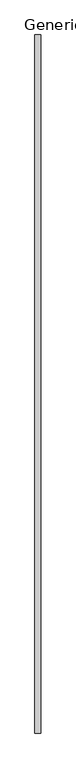
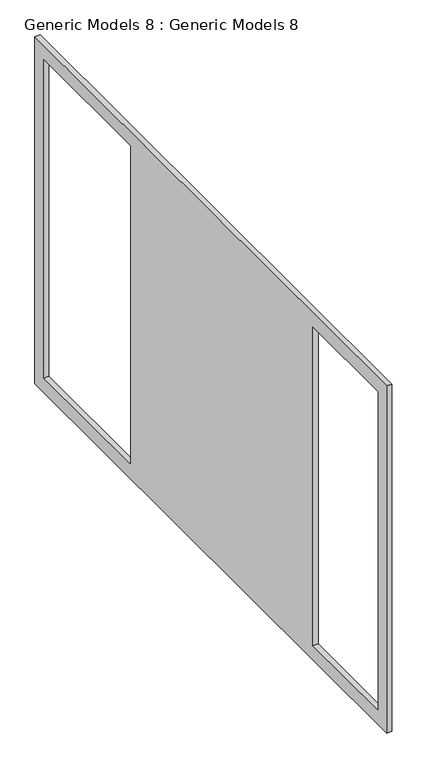
"""IFC4 building model written with IfcOpenShell, lengths in millimetres: proxy geometry, Generic Models 8 : Generic Models 8."""

from ifc_helpers import new_model, si_unit, frame, origin, place, context, project, spatial, polyline, outline, extrude, source, transform, mapped, element, save


def generic_models_8_generic_models_8_8aa07b80(model_context):
    return source(origin(), model_context, "Body", "SweptSolid", [
        extrude(outline(polyline([(152.4641252, 7010.4), (152.4641252, 3352.8), (-5918.1358748, 3352.8), (-5918.1358748, 7010.4), (152.4641252, 7010.4)]), holes=[polyline([(-4647.9588019, 6858.0), (-5765.7358748, 6858.0), (-5765.7358748, 3505.2), (-4647.9588019, 3505.2), (-4647.9588019, 6858.0)]), polyline([(-1492.6399037, 6858.0), (-1492.6399037, 3505.2), (0.0641252, 3505.2), (0.0641252, 6858.0), (-1492.6399037, 6858.0)])]), frame((4189.5719693, 0.0, 0.0), z_axis=(1.0, 0.0, 0.0), x_axis=(0.0, 1.0, 0.0)), (0.0, 0.0, 1.0), 50.8),
    ])


if __name__ == "__main__":
    model = new_model("IFC4")
    model_context = context("Model", 3, world=origin())
    ifc_project = project(units=[si_unit("LENGTHUNIT", "METRE", prefix="MILLI")], contexts=[model_context])
    site = spatial("IfcSite", under=ifc_project)
    building = spatial("IfcBuilding", under=site)
    placement = place(None, origin())
    generic_models_8_generic_models_8_shape = generic_models_8_generic_models_8_8aa07b80(model_context)
    element("IfcBuildingElementProxy", 1, Name="Generic Models 8 : Generic Models 8", ObjectType="Generic Models 8 : Generic Models 8", at=placement, inside=building, context=model_context, shape_type="MappedRepresentation", body=[
        mapped(generic_models_8_generic_models_8_shape, transform((0.0, 0.0, 0.0), x_axis=(1.0, 0.0, 0.0), y_axis=(0.0, 1.0, 0.0), z_axis=(0.0, 0.0, 1.0))),
    ])
    save(model, "model.ifc")

# Revit data of these elements
# Element 1 (IfcBuildingElementProxy, "Generic Models 8 : Generic Models 8")
#   Materials on its faces: "chocolate brown"
# Materials
#   "chocolate brown": class "Generic", colour RGB 120 120 120, transparency 0, Cost = 0
